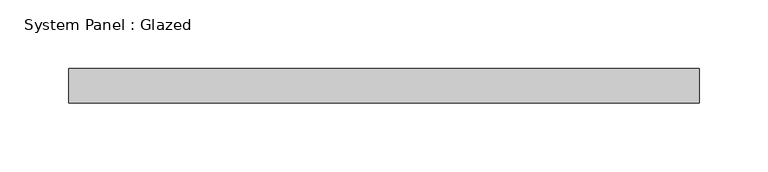
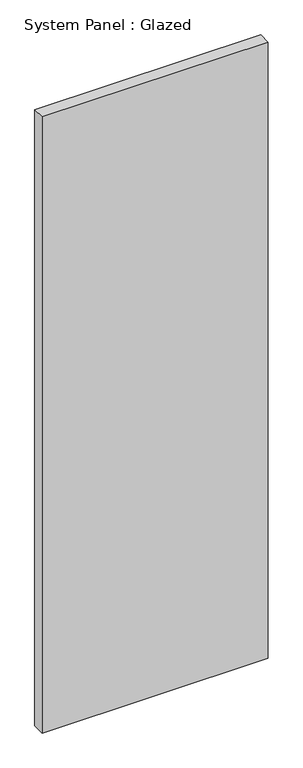
"""IFC4 building model written with IfcOpenShell, lengths in millimetres: plate geometry, System Panel : Glazed."""

from ifc_helpers import new_model, si_unit, origin, origin_with_axes, place, context, project, spatial, polyline, outline, extrude, source, transform, mapped, element, save


def system_panel_glazed_4e802334(model_context):
    return source(origin(), model_context, "Body", "SweptSolid", [
        extrude(outline(polyline([(230.1875, 19.05), (-230.1875, 19.05), (-230.1875, 44.45), (230.1875, 44.45), (230.1875, 19.05)])), origin_with_axes(), (0.0, 0.0, 1.0), 1325.5193485),
    ])


if __name__ == "__main__":
    model = new_model("IFC4")
    model_context = context("Model", 3, world=origin())
    ifc_project = project(units=[si_unit("LENGTHUNIT", "METRE", prefix="MILLI")], contexts=[model_context])
    site = spatial("IfcSite", under=ifc_project)
    building = spatial("IfcBuilding", under=site)
    placement = place(None, origin())
    system_panel_glazed_shape = system_panel_glazed_4e802334(model_context)
    element("IfcPlate", 1, ObjectType="System Panel : Glazed", at=placement, inside=building, context=model_context, shape_type="MappedRepresentation", body=[
        mapped(system_panel_glazed_shape, transform((0.0, 0.0, 0.0), x_axis=(1.0, 0.0, 0.0), y_axis=(0.0, 1.0, 0.0), z_axis=(0.0, 0.0, 1.0))),
    ])
    save(model, "model.ifc")

# Revit data of these elements
# Type "System Panel : Glazed"
#   Construction Type Id = "GSP4R"
#   Analytic Construction = "1/8 in Pilkington single glazing"
#   Visual Light Transmittance = 0.9
#   Solar Heat Gain Coefficient = 0.86
#   Heat Transfer Coefficient (U) = 1.18115 BTU/(h·ft²·°F)
#   Define Thermal Properties by = 1
# Element 1 (IfcPlate, "System Panel : Glazed")
#   Materials on its faces: "Glass"
# Materials
#   "Glass": class "Glass", colour RGB 0 128 192, transparency 0.75, Description = "Soda Lime Glass", Cost = 0
